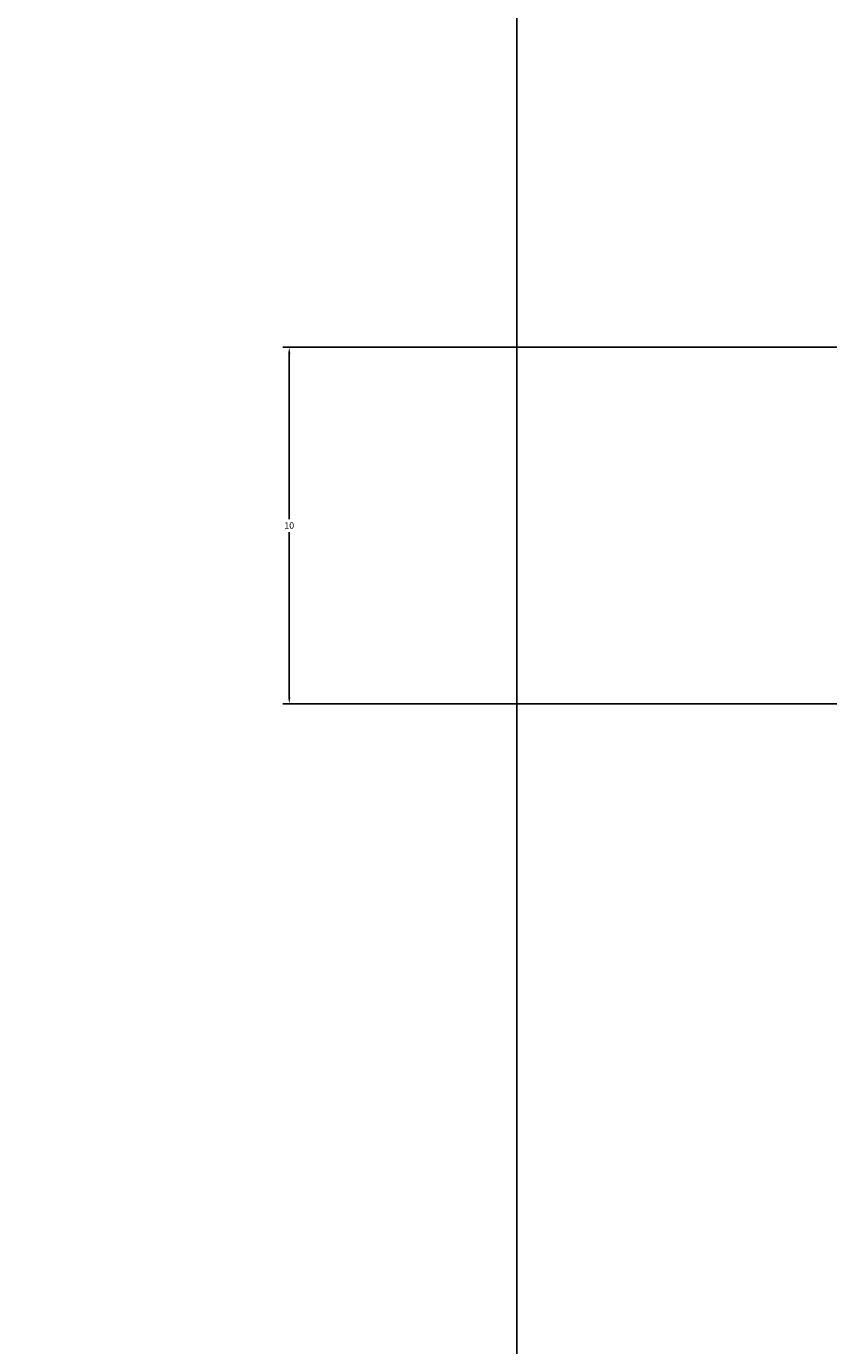
# Model space of a CAD drawing. Units: inches. Extents: x 2231 to 2461, y 2045 to 2455.
# Tile 61 of 95: x 2371 to 2393, y 2259 to 2296. Entities that reach past the tile are written whole.
import ezdxf

# ---------------------------------------------------------------- set-up
doc = ezdxf.new("R2010")
doc.units = ezdxf.units.IN
doc.layers.add('A-ANNO-DIMS', color=2, linetype='Continuous', lineweight=18)
doc.styles.get("Standard").update_dxf_attribs({"font": 'arial.ttf'})
doc.dimstyles.get("Standard").update_dxf_attribs({"dimtxt": 0.18, "dimasz": 0.18, "dimexe": 0.18, "dimexo": 0.0625, "dimgap": 0.09, "dimtad": 0, "dimtih": 1, "dimtoh": 1, "dimdec": 4, "dimzin": 0, "dimdsep": 46, "dimtxsty": 'Standard', "dimcen": 0.09, "dimadec": 0, "dimazin": 0, "dimtfac": 1, "dimtdec": 4, "dimtofl": 0, "dimtmove": 0, "dimatfit": 3, "dimfxl": 1, "dimtolj": 1, "dimtzin": 0, "dimarcsym": 0})

# ---------------------------------------------------------------- blocks, each defined once
blk = doc.blocks.new('*D66')
at = {"layer": 'A-ANNO-DIMS', "color": 0, "lineweight": -2, "transparency": 16777216}
for p, q in [((2348.189, 2096.895), (2348.189, 2454.645)), ((2408.794, 2096.895), (2408.794, 2454.645)), ((2348.369, 2454.465), (2378.167, 2454.465)), ((2408.614, 2454.465), (2378.815, 2454.465))]:
    blk.add_line(p, q, dxfattribs=at)
at = {"layer": 'A-ANNO-DIMS', "color": 0, "transparency": 16777216}
for points in [[(2348.369, 2454.495), (2348.369, 2454.435), (2348.189, 2454.465)], [(2408.614, 2454.495), (2408.614, 2454.435), (2408.794, 2454.465)]]:
    blk.add_solid(points, dxfattribs=at)
at = {"layer": 'Defpoints', "color": 0, "transparency": 16777216}
for p in [(2408.794, 2454.465), (2348.189, 2096.833), (2408.794, 2096.833)]:
    blk.add_point(p, dxfattribs=at)
at = {"layer": 'A-ANNO-DIMS', "color": 0, "transparency": 16777216, "insert": (2378.491, 2454.465), "char_height": 0.18, "attachment_point": 5}
blk.add_mtext('\\A1;60.6', dxfattribs=at)
blk = doc.blocks.new('*D72')
at = {"layer": 'A-ANNO-DIMS', "color": 0, "lineweight": -2, "transparency": 16777216}
for p, q in [((2384.543, 2145.12), (2384.543, 2454.645)), ((2408.794, 2150.677), (2408.794, 2454.645)), ((2384.723, 2454.465), (2396.272, 2454.465)), ((2408.614, 2454.465), (2397.064, 2454.465))]:
    blk.add_line(p, q, dxfattribs=at)
at = {"layer": 'A-ANNO-DIMS', "color": 0, "transparency": 16777216}
for points in [[(2384.723, 2454.495), (2384.723, 2454.435), (2384.543, 2454.465)], [(2408.614, 2454.495), (2408.614, 2454.435), (2408.794, 2454.465)]]:
    blk.add_solid(points, dxfattribs=at)
at = {"layer": 'Defpoints', "color": 0, "transparency": 16777216}
for p in [(2408.794, 2454.465), (2408.794, 2150.615), (2384.543, 2145.058)]:
    blk.add_point(p, dxfattribs=at)
at = {"layer": 'A-ANNO-DIMS', "color": 0, "transparency": 16777216, "insert": (2396.668, 2454.465), "char_height": 0.18, "attachment_point": 5}
blk.add_mtext('\\A1;24.25', dxfattribs=at)
blk = doc.blocks.new('*D74')
at = {"layer": 'A-ANNO-DIMS', "color": 0, "lineweight": -2, "transparency": 16777216}
for p, q in [((2396.731, 2286.833), (2377.981, 2286.833)), ((2378.161, 2286.653), (2378.161, 2282.015)), ((2378.161, 2277.013), (2378.161, 2281.651)), ((2396.731, 2276.833), (2377.981, 2276.833))]:
    blk.add_line(p, q, dxfattribs=at)
at = {"layer": 'A-ANNO-DIMS', "color": 0, "transparency": 16777216}
for points in [[(2378.131, 2286.653), (2378.191, 2286.653), (2378.161, 2286.833)], [(2378.131, 2277.013), (2378.191, 2277.013), (2378.161, 2276.833)]]:
    blk.add_solid(points, dxfattribs=at)
at = {"layer": 'Defpoints', "color": 0, "transparency": 16777216}
for p in [(2378.161, 2286.833), (2396.794, 2286.833), (2396.794, 2276.833)]:
    blk.add_point(p, dxfattribs=at)
at = {"layer": 'A-ANNO-DIMS', "color": 0, "transparency": 16777216, "insert": (2378.161, 2281.833), "char_height": 0.18, "attachment_point": 5}
blk.add_mtext('\\A1;10', dxfattribs=at)

msp = doc.modelspace()

# ---------------------------------------------------------------- dimensions: what is measured, and where the dimension line sits
at = {"layer": 'A-ANNO-DIMS'}
for p1, p2, override, picture, middle in [((2348.1888, 2096.8328), (2408.7935, 2096.8328), {"dimdec": 1, "dimlfac": 1, "dimrnd": 0, "dimzin": 0, "dimdsep": 46, "dimlunit": 2}, '*D66', (2378.4912, 2454.4653)), ((2384.5428, 2145.0576), (2408.7935, 2150.6145), {"dimdec": 2, "dimlfac": 1, "dimrnd": 0, "dimzin": 0, "dimdsep": 46, "dimlunit": 2}, '*D72', (2396.6682, 2454.4653))]:
    dim = msp.add_linear_dim(base=(2408.7935, 2454.4653), p1=p1, p2=p2, dimstyle='Standard', override=override, dxfattribs=at)
    dim.commit()
    dim.dimension.update_dxf_attribs({"geometry": picture, "text_midpoint": middle})
dim = msp.add_linear_dim(base=(2378.161, 2286.8328), p1=(2396.7935, 2276.8328), p2=(2396.7935, 2286.8328), angle=90, dimstyle='Standard', override={"dimdec": 0, "dimlfac": 1, "dimrnd": 0, "dimzin": 0, "dimdsep": 46, "dimlunit": 2}, dxfattribs=at)
dim.commit()
dim.dimension.update_dxf_attribs({"geometry": '*D74', "text_midpoint": (2378.161, 2281.8328)})

doc.saveas('drawing.dxf')
